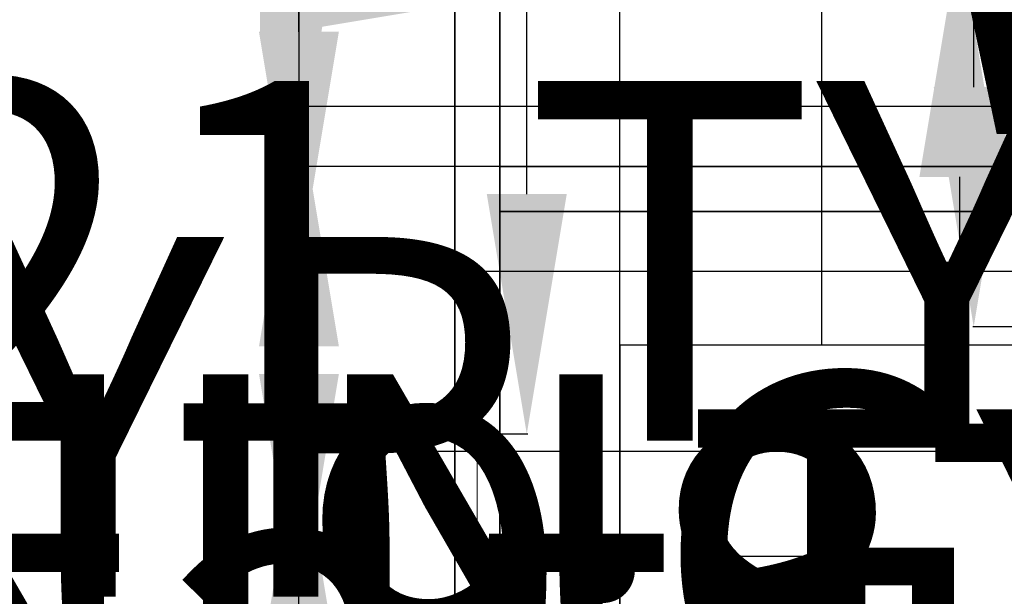
# Model space of a CAD drawing. Units: inches. Extents: x -307 to 2141, y -58 to 895.
# Tile 10 of 28: x 469 to 666, y 452 to 568. Entities that reach past the tile are written whole.
import ezdxf

# ---------------------------------------------------------------- set-up
doc = ezdxf.new("R2010")
doc.units = ezdxf.units.IN
doc.header["$MEASUREMENT"] = 0
for name, color, linetype, lineweight in [('A-ANNO-DIMS', 2, 'Continuous', 18), ('A-DOOR', 3, 'Continuous', 25), ('A-FLOR-CASE', 32, 'Continuous', 25), ('A-GLAZ', 4, 'Continuous', 18), ('A-WALL', 7, 'Continuous', 35)]:
    doc.layers.add(name, color=color, linetype=linetype, lineweight=lineweight)
doc.styles.get("Standard").update_dxf_attribs({"font": 'arial.ttf'})
doc.dimstyles.get("Standard").update_dxf_attribs({"dimtxt": 72, "dimasz": 48, "dimexe": 0.18, "dimexo": 0.0625, "dimgap": 0.09, "dimtad": 0, "dimtih": 1, "dimtoh": 1, "dimdec": 0, "dimrnd": 48, "dimzin": 0, "dimdsep": 46, "dimlunit": 3, "dimtxsty": 'Standard', "dimcen": 0.09, "dimadec": 0, "dimazin": 0, "dimtfac": 1, "dimtdec": 0, "dimtofl": 0, "dimtmove": 0, "dimatfit": 3, "dimfxl": 1, "dimtolj": 1, "dimtzin": 0, "dimarcsym": 0})

# ---------------------------------------------------------------- blocks, each defined once
blk = doc.blocks.new('*U3')
for p, q in [((-40, 0), (-40, 6)), ((0, 0), (0, 6))]:
    blk.add_line(p, q)
blk.add_lwpolyline([(0, 0), (-34.64, -20), (-35.52, -18.48), (-0.88, 1.52)], close=True)
blk.add_arc((0, 0), 40, 180, 210)
blk = doc.blocks.new('WIN-36IN')
for p, q in [((0, 36), (9, 36)), ((4.5, 0), (4.5, 36))]:
    blk.add_line(p, q)
blk.add_lwpolyline([(9, 36), (9, 0), (0, 0), (0, 36)])
blk = doc.blocks.new('*D26')
at = {"layer": 'A-ANNO-DIMS', "color": 0, "lineweight": -2, "transparency": 16777216}
for p, q in [((565.34, 584.2), (565.34, 572.08)), ((645.34, 584.2), (645.34, 572.08)), ((517.34, 572.26), (469.34, 572.26)), ((693.34, 572.26), (741.34, 572.26))]:
    blk.add_line(p, q, dxfattribs=at)
at = {"layer": 'A-ANNO-DIMS', "color": 0, "transparency": 16777216}
for points in [[(517.34, 580.26), (517.34, 564.26), (565.34, 572.26)], [(693.34, 580.26), (693.34, 564.26), (645.34, 572.26)]]:
    blk.add_solid(points, dxfattribs=at)
at = {"layer": 'Defpoints', "color": 0, "transparency": 16777216}
for p in [(565.34, 584.26), (645.34, 584.26), (565.34, 572.26)]:
    blk.add_point(p, dxfattribs=at)
at = {"layer": 'A-ANNO-DIMS', "color": 0, "transparency": 16777216, "insert": (178.23, 572.26), "char_height": 72, "attachment_point": 5}
blk.add_mtext('\\A1;BED 80 TYP.', dxfattribs=at)
blk = doc.blocks.new('*D27')
at = {"layer": 'A-ANNO-DIMS', "color": 0, "lineweight": -2, "transparency": 16777216}
for p, q in [((657.34, 692.26), (657.34, 740.26)), ((645.4, 644.26), (657.52, 644.26)), ((645.4, 584.26), (657.52, 584.26)), ((657.34, 536.26), (657.34, 488.26)), ((657.34, 488.26), (609.34, 488.26))]:
    blk.add_line(p, q, dxfattribs=at)
at = {"layer": 'A-ANNO-DIMS', "color": 0, "transparency": 16777216}
for points in [[(649.34, 692.26), (665.34, 692.26), (657.34, 644.26)], [(649.34, 536.26), (665.34, 536.26), (657.34, 584.26)]]:
    blk.add_solid(points, dxfattribs=at)
at = {"layer": 'Defpoints', "color": 0, "transparency": 16777216}
for p in [(645.34, 644.26), (645.34, 584.26), (657.34, 584.26)]:
    blk.add_point(p, dxfattribs=at)
at = {"layer": 'A-ANNO-DIMS', "color": 0, "transparency": 16777216, "insert": (433.81, 488.26), "char_height": 72, "attachment_point": 5}
blk.add_mtext('\\A1;60 TYP.', dxfattribs=at)
blk = doc.blocks.new('*D29')
at = {"layer": 'A-ANNO-DIMS', "color": 0, "lineweight": -2, "transparency": 16777216}
for p, q in [((747.42, 450.87), (699.42, 450.87)), ((795.42, 433.61), (795.42, 451.05)), ((882.03, 433.61), (882.03, 451.05)), ((930.03, 450.87), (978.03, 450.87))]:
    blk.add_line(p, q, dxfattribs=at)
at = {"layer": 'A-ANNO-DIMS', "color": 0, "transparency": 16777216}
for points in [[(747.42, 458.87), (747.42, 442.87), (795.42, 450.87)], [(930.03, 458.87), (930.03, 442.87), (882.03, 450.87)]]:
    blk.add_solid(points, dxfattribs=at)
at = {"layer": 'Defpoints', "color": 0, "transparency": 16777216}
for p in [(795.42, 450.87), (795.42, 433.55), (882.03, 433.55)]:
    blk.add_point(p, dxfattribs=at)
at = {"layer": 'A-ANNO-DIMS', "color": 0, "transparency": 16777216, "insert": (647.71, 450.87), "char_height": 72, "attachment_point": 5}
blk.add_mtext('\\A1;87', dxfattribs=at)
blk = doc.blocks.new('*D30')
at = {"layer": 'A-ANNO-DIMS', "color": 0, "lineweight": -2, "transparency": 16777216}
for p, q in [((570.74, 532.83), (570.74, 580.83)), ((570.74, 580.83), (618.74, 580.83)), ((565.4, 484.83), (570.92, 484.83)), ((565.4, 448.83), (570.92, 448.83)), ((570.74, 400.83), (570.74, 352.83))]:
    blk.add_line(p, q, dxfattribs=at)
at = {"layer": 'A-ANNO-DIMS', "color": 0, "transparency": 16777216}
for points in [[(562.74, 532.83), (578.74, 532.83), (570.74, 484.83)], [(562.74, 400.83), (578.74, 400.83), (570.74, 448.83)]]:
    blk.add_solid(points, dxfattribs=at)
at = {"layer": 'Defpoints', "color": 0, "transparency": 16777216}
for p in [(565.34, 484.83), (570.74, 484.83), (565.34, 448.83)]:
    blk.add_point(p, dxfattribs=at)
at = {"layer": 'A-ANNO-DIMS', "color": 0, "transparency": 16777216, "insert": (1030.17, 580.83), "char_height": 72, "attachment_point": 5}
blk.add_mtext('\\A1;WINDOW 36 TYP.', dxfattribs=at)
blk = doc.blocks.new('*D31')
at = {"layer": 'A-ANNO-DIMS', "color": 0, "lineweight": -2, "transparency": 16777216}
for p, q in [((556.34, 448.77), (556.34, 443.25)), ((565.34, 448.77), (565.34, 443.25)), ((508.34, 443.43), (460.34, 443.43)), ((613.34, 443.43), (661.34, 443.43))]:
    blk.add_line(p, q, dxfattribs=at)
at = {"layer": 'A-ANNO-DIMS', "color": 0, "transparency": 16777216}
for points in [[(508.34, 451.43), (508.34, 435.43), (556.34, 443.43)], [(613.34, 451.43), (613.34, 435.43), (565.34, 443.43)]]:
    blk.add_solid(points, dxfattribs=at)
at = {"layer": 'Defpoints', "color": 0, "transparency": 16777216}
for p in [(556.34, 448.83), (565.34, 448.83), (565.34, 443.43)]:
    blk.add_point(p, dxfattribs=at)
at = {"layer": 'A-ANNO-DIMS', "color": 0, "transparency": 16777216, "insert": (808.69, 443.43), "char_height": 72, "attachment_point": 5}
blk.add_mtext('\\A1;9 TYP.', dxfattribs=at)
blk = doc.blocks.new('*D35')
at = {"layer": 'A-ANNO-DIMS', "color": 0, "lineweight": -2, "transparency": 16777216}
for p, q in [((859.34, 453.77), (811.34, 453.77)), ((907.34, 443.03), (907.34, 453.95)), ((916.34, 443.03), (916.34, 453.95)), ((964.34, 453.77), (1012.34, 453.77))]:
    blk.add_line(p, q, dxfattribs=at)
at = {"layer": 'A-ANNO-DIMS', "color": 0, "transparency": 16777216}
for points in [[(859.34, 461.77), (859.34, 445.77), (907.34, 453.77)], [(964.34, 461.77), (964.34, 445.77), (916.34, 453.77)]]:
    blk.add_solid(points, dxfattribs=at)
at = {"layer": 'Defpoints', "color": 0, "transparency": 16777216}
for p in [(907.34, 453.77), (907.34, 442.97), (916.34, 442.97)]:
    blk.add_point(p, dxfattribs=at)
at = {"layer": 'A-ANNO-DIMS', "color": 0, "transparency": 16777216, "insert": (663.98, 453.77), "char_height": 72, "attachment_point": 5}
blk.add_mtext('\\A1;9 TYP.', dxfattribs=at)
blk = doc.blocks.new('*D36')
at = {"layer": 'A-ANNO-DIMS', "color": 0, "lineweight": -2, "transparency": 16777216}
for p, q in [((871.71, 562.4), (871.76, 610.4)), ((876.55, 514.4), (871.47, 514.4)), ((876.51, 481.35), (871.44, 481.36)), ((871.56, 433.36), (871.51, 385.36)), ((871.51, 385.36), (823.51, 385.36))]:
    blk.add_line(p, q, dxfattribs=at)
at = {"layer": 'A-ANNO-DIMS', "color": 0, "transparency": 16777216}
for points in [[(863.71, 562.41), (879.71, 562.4), (871.65, 514.4)], [(863.56, 433.37), (879.56, 433.35), (871.62, 481.36)]]:
    blk.add_solid(points, dxfattribs=at)
at = {"layer": 'Defpoints', "color": 0, "transparency": 16777216}
for p in [(876.61, 514.4), (871.62, 481.36), (876.57, 481.35)]:
    blk.add_point(p, dxfattribs=at)
at = {"layer": 'A-ANNO-DIMS', "color": 0, "transparency": 16777216, "insert": (548.95, 385.36), "char_height": 72, "attachment_point": 5}
blk.add_mtext('\\A1;WC 33 TYP.', dxfattribs=at)
blk = doc.blocks.new('*D37')
at = {"layer": 'A-ANNO-DIMS', "color": 0, "lineweight": -2, "transparency": 16777216}
for p, q in [((828.62, 519.41), (780.62, 519.46)), ((876.61, 514.46), (876.62, 519.54)), ((897.61, 514.44), (897.62, 519.51)), ((945.62, 519.28), (993.62, 519.22))]:
    blk.add_line(p, q, dxfattribs=at)
at = {"layer": 'A-ANNO-DIMS', "color": 0, "transparency": 16777216}
for points in [[(828.63, 527.41), (828.61, 511.41), (876.62, 519.36)], [(945.63, 527.28), (945.61, 511.28), (897.62, 519.33)]]:
    blk.add_solid(points, dxfattribs=at)
at = {"layer": 'Defpoints', "color": 0, "transparency": 16777216}
for p in [(876.62, 519.36), (876.61, 514.4), (897.61, 514.38)]:
    blk.add_point(p, dxfattribs=at)
at = {"layer": 'A-ANNO-DIMS', "color": 0, "transparency": 16777216, "insert": (604.68, 519.46), "char_height": 72, "attachment_point": 5}
blk.add_mtext('\\A1;21 TYP.', dxfattribs=at)
blk = doc.blocks.new('*D51')
at = {"layer": 'A-ANNO-DIMS', "color": 0, "lineweight": -2, "transparency": 16777216}
for p, q in [((562.8, 379.11), (562.8, 427.11)), ((562.8, 427.11), (610.8, 427.11)), ((565.27, 331.11), (562.62, 331.11)), ((565.27, 315.87), (562.62, 315.87)), ((562.8, 267.87), (562.8, 219.87))]:
    blk.add_line(p, q, dxfattribs=at)
at = {"layer": 'A-ANNO-DIMS', "color": 0, "transparency": 16777216}
for points in [[(554.8, 379.11), (570.8, 379.11), (562.8, 331.11)], [(554.8, 267.87), (570.8, 267.87), (562.8, 315.87)]]:
    blk.add_solid(points, dxfattribs=at)
at = {"layer": 'Defpoints', "color": 0, "transparency": 16777216}
for p in [(562.8, 331.11), (565.34, 331.11), (565.34, 315.87)]:
    blk.add_point(p, dxfattribs=at)
at = {"layer": 'A-ANNO-DIMS', "color": 0, "transparency": 16777216, "insert": (659.34, 427.11), "char_height": 72, "attachment_point": 5}
blk.add_mtext('\\A1;15', dxfattribs=at)
blk = doc.blocks.new('*D52')
at = {"layer": 'A-ANNO-DIMS', "color": 0, "lineweight": -2, "transparency": 16777216}
for p, q in [((660.21, 554.25), (660.21, 602.25)), ((673.8, 506.25), (660.03, 506.25)), ((673.8, 415.25), (660.03, 415.25)), ((660.21, 367.25), (660.21, 319.25))]:
    blk.add_line(p, q, dxfattribs=at)
at = {"layer": 'A-ANNO-DIMS', "color": 0, "transparency": 16777216}
for points in [[(652.21, 554.25), (668.21, 554.25), (660.21, 506.25)], [(652.21, 367.25), (668.21, 367.25), (660.21, 415.25)]]:
    blk.add_solid(points, dxfattribs=at)
at = {"layer": 'Defpoints', "color": 0, "transparency": 16777216}
for p in [(673.86, 506.25), (660.21, 415.25), (673.86, 415.25)]:
    blk.add_point(p, dxfattribs=at)
at = {"layer": 'A-ANNO-DIMS', "color": 0, "transparency": 16777216, "insert": (660.21, 460.75), "char_height": 72, "attachment_point": 5}
blk.add_mtext('\\A1;DINING SET 91', dxfattribs=at)
blk = doc.blocks.new('*D54')
at = {"layer": 'A-ANNO-DIMS', "color": 0, "lineweight": -2, "transparency": 16777216}
for p, q in [((605.34, 412.35), (605.34, 460.35)), ((605.34, 460.35), (653.34, 460.35)), ((596.4, 364.35), (605.52, 364.35)), ((596.4, 304.35), (605.52, 304.35)), ((605.34, 256.35), (605.34, 208.35))]:
    blk.add_line(p, q, dxfattribs=at)
at = {"layer": 'A-ANNO-DIMS', "color": 0, "transparency": 16777216}
for points in [[(597.34, 412.35), (613.34, 412.35), (605.34, 364.35)], [(597.34, 256.35), (613.34, 256.35), (605.34, 304.35)]]:
    blk.add_solid(points, dxfattribs=at)
at = {"layer": 'Defpoints', "color": 0, "transparency": 16777216}
for p in [(596.34, 364.35), (605.34, 364.35), (596.34, 304.35)]:
    blk.add_point(p, dxfattribs=at)
at = {"layer": 'A-ANNO-DIMS', "color": 0, "transparency": 16777216, "insert": (854, 460.35), "char_height": 72, "attachment_point": 5}
blk.add_mtext('\\A1;DESK 60', dxfattribs=at)
blk = doc.blocks.new('*D62')
at = {"layer": 'A-ANNO-DIMS', "color": 0, "lineweight": -2, "transparency": 16777216}
for p, q in [((556.34, 691.4), (556.34, 722.72)), ((604.34, 722.54), (656.85, 722.54)), ((868.34, 722.54), (815.82, 722.54)), ((916.34, 490.97), (916.34, 722.72))]:
    blk.add_line(p, q, dxfattribs=at)
at = {"layer": 'A-ANNO-DIMS', "color": 0, "transparency": 16777216}
for points in [[(604.34, 730.54), (604.34, 714.54), (556.34, 722.54)], [(868.34, 730.54), (868.34, 714.54), (916.34, 722.54)]]:
    blk.add_solid(points, dxfattribs=at)
at = {"layer": 'Defpoints', "color": 0, "transparency": 16777216}
for p in [(916.34, 722.54), (556.34, 691.34), (916.34, 490.9)]:
    blk.add_point(p, dxfattribs=at)
at = {"layer": 'A-ANNO-DIMS', "color": 0, "transparency": 16777216, "insert": (736.34, 722.54), "char_height": 72, "attachment_point": 5}
blk.add_mtext('\\A1;360', dxfattribs=at)
blk = doc.blocks.new('*D64')
at = {"layer": 'A-ANNO-DIMS', "color": 0, "lineweight": -2, "transparency": 16777216}
for p, q in [((556.27, 691.34), (524.95, 691.34)), ((525.13, 643.34), (525.13, 465.69)), ((525.13, 214.34), (525.13, 391.99)), ((556.27, 166.34), (524.95, 166.34))]:
    blk.add_line(p, q, dxfattribs=at)
at = {"layer": 'A-ANNO-DIMS', "color": 0, "transparency": 16777216}
for points in [[(517.13, 643.34), (533.13, 643.34), (525.13, 691.34)], [(517.13, 214.34), (533.13, 214.34), (525.13, 166.34)]]:
    blk.add_solid(points, dxfattribs=at)
at = {"layer": 'Defpoints', "color": 0, "transparency": 16777216}
for p in [(525.13, 691.34), (556.34, 691.34), (556.34, 166.34)]:
    blk.add_point(p, dxfattribs=at)
at = {"layer": 'A-ANNO-DIMS', "color": 0, "transparency": 16777216, "insert": (525.13, 428.84), "char_height": 72, "attachment_point": 5}
blk.add_mtext('\\A1;525', dxfattribs=at)
blk = doc.blocks.new('*D67')
at = {"layer": 'A-ANNO-DIMS', "color": 0, "lineweight": -2, "transparency": 16777216}
for p, q in [((525.13, 496.83), (525.13, 544.83)), ((556.27, 448.83), (524.95, 448.83)), ((556.27, 370.34), (524.95, 370.34)), ((525.13, 322.34), (525.13, 274.34))]:
    blk.add_line(p, q, dxfattribs=at)
at = {"layer": 'A-ANNO-DIMS', "color": 0, "transparency": 16777216}
for points in [[(517.13, 496.83), (533.13, 496.83), (525.13, 448.83)], [(517.13, 322.34), (533.13, 322.34), (525.13, 370.34)]]:
    blk.add_solid(points, dxfattribs=at)
at = {"layer": 'Defpoints', "color": 0, "transparency": 16777216}
for p in [(525.13, 448.83), (556.34, 448.83), (556.34, 370.34)]:
    blk.add_point(p, dxfattribs=at)
at = {"layer": 'A-ANNO-DIMS', "color": 0, "transparency": 16777216, "insert": (525.13, 409.59), "char_height": 72, "attachment_point": 5}
blk.add_mtext('\\A1;78.49', dxfattribs=at)
blk = doc.blocks.new('*D68')
at = {"layer": 'A-ANNO-DIMS', "color": 0, "lineweight": -2, "transparency": 16777216}
for p, q in [((525.13, 586.34), (525.13, 634.34)), ((525.13, 634.34), (573.13, 634.34)), ((565.27, 538.34), (524.95, 538.34)), ((556.27, 484.83), (524.95, 484.83)), ((525.13, 436.83), (525.13, 388.83))]:
    blk.add_line(p, q, dxfattribs=at)
at = {"layer": 'A-ANNO-DIMS', "color": 0, "transparency": 16777216}
for points in [[(517.13, 586.34), (533.13, 586.34), (525.13, 538.34)], [(517.13, 436.83), (533.13, 436.83), (525.13, 484.83)]]:
    blk.add_solid(points, dxfattribs=at)
at = {"layer": 'Defpoints', "color": 0, "transparency": 16777216}
for p in [(525.13, 538.34), (565.34, 538.34), (556.34, 484.83)]:
    blk.add_point(p, dxfattribs=at)
at = {"layer": 'A-ANNO-DIMS', "color": 0, "transparency": 16777216, "insert": (687.75, 634.34), "char_height": 72, "attachment_point": 5}
blk.add_mtext('\\A1;53.51', dxfattribs=at)
blk = doc.blocks.new('*D69')
at = {"layer": 'A-ANNO-DIMS', "color": 0, "lineweight": -2, "transparency": 16777216}
for p, q in [((525.13, 682.34), (525.13, 730.34)), ((525.13, 730.34), (573.13, 730.34)), ((565.27, 682.34), (524.95, 682.34)), ((525.13, 586.34), (525.13, 634.34)), ((565.27, 538.34), (524.95, 538.34))]:
    blk.add_line(p, q, dxfattribs=at)
at = {"layer": 'A-ANNO-DIMS', "color": 0, "transparency": 16777216}
for points in [[(517.13, 634.34), (533.13, 634.34), (525.13, 682.34)], [(517.13, 586.34), (533.13, 586.34), (525.13, 538.34)]]:
    blk.add_solid(points, dxfattribs=at)
at = {"layer": 'Defpoints', "color": 0, "transparency": 16777216}
for p in [(525.13, 682.34), (565.34, 682.34), (565.34, 538.34)]:
    blk.add_point(p, dxfattribs=at)
at = {"layer": 'A-ANNO-DIMS', "color": 0, "transparency": 16777216, "insert": (649.22, 730.34), "char_height": 72, "attachment_point": 5}
blk.add_mtext('\\A1;144', dxfattribs=at)
blk = doc.blocks.new('*D82')
at = {"layer": 'A-ANNO-DIMS', "color": 0, "lineweight": -2, "transparency": 16777216}
for p, q in [((525.13, 565.34), (525.13, 613.34)), ((525.13, 613.34), (573.13, 613.34)), ((802.27, 517.34), (524.95, 517.34)), ((802.27, 481.34), (524.95, 481.34)), ((525.13, 433.34), (525.13, 385.34))]:
    blk.add_line(p, q, dxfattribs=at)
at = {"layer": 'A-ANNO-DIMS', "color": 0, "transparency": 16777216}
for points in [[(517.13, 565.34), (533.13, 565.34), (525.13, 517.34)], [(517.13, 433.34), (533.13, 433.34), (525.13, 481.34)]]:
    blk.add_solid(points, dxfattribs=at)
at = {"layer": 'Defpoints', "color": 0, "transparency": 16777216}
for p in [(525.13, 517.34), (802.34, 517.34), (802.34, 481.34)]:
    blk.add_point(p, dxfattribs=at)
at = {"layer": 'A-ANNO-DIMS', "color": 0, "transparency": 16777216, "insert": (624.74, 613.34), "char_height": 72, "attachment_point": 5}
blk.add_mtext('\\A1;36', dxfattribs=at)
blk = doc.blocks.new('*D83')
at = {"layer": 'A-ANNO-DIMS', "color": 0, "lineweight": -2, "transparency": 16777216}
for p, q in [((947.54, 538.9), (947.54, 586.9)), ((916.4, 490.9), (947.72, 490.9)), ((907.4, 481.34), (947.72, 481.34)), ((947.54, 433.34), (947.54, 385.34)), ((947.54, 385.34), (899.54, 385.34))]:
    blk.add_line(p, q, dxfattribs=at)
at = {"layer": 'A-ANNO-DIMS', "color": 0, "transparency": 16777216}
for points in [[(939.54, 538.9), (955.54, 538.9), (947.54, 490.9)], [(939.54, 433.34), (955.54, 433.34), (947.54, 481.34)]]:
    blk.add_solid(points, dxfattribs=at)
at = {"layer": 'Defpoints', "color": 0, "transparency": 16777216}
for p in [(916.34, 490.9), (907.34, 481.34), (947.54, 481.34)]:
    blk.add_point(p, dxfattribs=at)
at = {"layer": 'A-ANNO-DIMS', "color": 0, "transparency": 16777216, "insert": (777.97, 385.34), "char_height": 72, "attachment_point": 5}
blk.add_mtext('\\A1;9.563', dxfattribs=at)
blk = doc.blocks.new('*D87')
at = {"layer": 'A-ANNO-DIMS', "color": 0, "lineweight": -2, "transparency": 16777216}
for p, q in [((525.13184, 448.340828), (525.13184, 496.340828)), ((625.27334, 400.340828), (524.95184, 400.340828)), ((625.27334, 304.340828), (524.95184, 304.340828)), ((525.13184, 256.340828), (525.13184, 208.340828))]:
    blk.add_line(p, q, dxfattribs=at)
at = {"layer": 'A-ANNO-DIMS', "color": 0, "transparency": 16777216}
for points in [[(517.13184, 448.340828), (533.13184, 448.340828), (525.13184, 400.340828)], [(517.13184, 256.340828), (533.13184, 256.340828), (525.13184, 304.340828)]]:
    blk.add_solid(points, dxfattribs=at)
at = {"layer": 'Defpoints', "color": 0, "transparency": 16777216}
for p in [(525.13184, 400.340828), (625.33584, 400.340828), (625.33584, 304.340828)]:
    blk.add_point(p, dxfattribs=at)
at = {"layer": 'A-ANNO-DIMS', "color": 0, "transparency": 16777216, "insert": (525.13184, 352.340828), "char_height": 72, "attachment_point": 5}
blk.add_mtext('\\A1;96', dxfattribs=at)
blk = doc.blocks.new('*D88')
at = {"layer": 'A-ANNO-DIMS', "color": 0, "lineweight": -2, "transparency": 16777216}
for p, q in [((517.33584, 722.544828), (469.33584, 722.544828)), ((565.33584, 295.403328), (565.33584, 722.724828)), ((754.33584, 271.403328), (754.33584, 722.724828)), ((802.33584, 722.544828), (850.33584, 722.544828))]:
    blk.add_line(p, q, dxfattribs=at)
at = {"layer": 'A-ANNO-DIMS', "color": 0, "transparency": 16777216}
for points in [[(517.33584, 730.544828), (517.33584, 714.544828), (565.33584, 722.544828)], [(802.33584, 730.544828), (802.33584, 714.544828), (754.33584, 722.544828)]]:
    blk.add_solid(points, dxfattribs=at)
at = {"layer": 'Defpoints', "color": 0, "transparency": 16777216}
for p in [(754.33584, 722.544828), (565.33584, 295.340828), (754.33584, 271.340828)]:
    blk.add_point(p, dxfattribs=at)
at = {"layer": 'A-ANNO-DIMS', "color": 0, "transparency": 16777216, "insert": (659.83584, 722.544828), "char_height": 72, "attachment_point": 5}
blk.add_mtext('\\A1;189', dxfattribs=at)
blk = doc.blocks.new('*D94')
at = {"layer": 'A-ANNO-DIMS', "color": 0, "lineweight": -2, "transparency": 16777216}
for p, q in [((517.34, 722.54), (469.34, 722.54)), ((565.34, 529.4), (565.34, 722.72)), ((629.84, 529.4), (629.84, 722.72)), ((677.84, 722.54), (725.84, 722.54))]:
    blk.add_line(p, q, dxfattribs=at)
at = {"layer": 'A-ANNO-DIMS', "color": 0, "transparency": 16777216}
for points in [[(517.34, 730.54), (517.34, 714.54), (565.34, 722.54)], [(677.84, 730.54), (677.84, 714.54), (629.84, 722.54)]]:
    blk.add_solid(points, dxfattribs=at)
at = {"layer": 'Defpoints', "color": 0, "transparency": 16777216}
for p in [(629.84, 722.54), (565.34, 529.34), (629.84, 529.34)]:
    blk.add_point(p, dxfattribs=at)
at = {"layer": 'A-ANNO-DIMS', "color": 0, "transparency": 16777216, "insert": (819.9, 722.54), "char_height": 72, "attachment_point": 5}
blk.add_mtext('\\A1;64.5', dxfattribs=at)
blk = doc.blocks.new('*D95')
at = {"layer": 'A-ANNO-DIMS', "color": 0, "lineweight": -2, "transparency": 16777216}
for p, q in [((947.54, 577.34), (947.54, 625.34)), ((947.54, 625.34), (995.54, 625.34)), ((629.9, 529.34), (947.72, 529.34)), ((629.9, 502.66), (947.72, 502.66)), ((947.54, 454.66), (947.54, 406.66))]:
    blk.add_line(p, q, dxfattribs=at)
at = {"layer": 'A-ANNO-DIMS', "color": 0, "transparency": 16777216}
for points in [[(939.54, 577.34), (955.54, 577.34), (947.54, 529.34)], [(939.54, 454.66), (955.54, 454.66), (947.54, 502.66)]]:
    blk.add_solid(points, dxfattribs=at)
at = {"layer": 'Defpoints', "color": 0, "transparency": 16777216}
for p in [(629.84, 529.34), (947.54, 529.34), (629.84, 502.66)]:
    blk.add_point(p, dxfattribs=at)
at = {"layer": 'A-ANNO-DIMS', "color": 0, "transparency": 16777216, "insert": (1117.8, 625.34), "char_height": 72, "attachment_point": 5}
blk.add_mtext('\\A1;26.68', dxfattribs=at)
blk = doc.blocks.new('*D98')
at = {"layer": 'A-ANNO-DIMS', "color": 0, "lineweight": -2, "transparency": 16777216}
for p, q in [((525.13, 637.34), (525.13, 685.34)), ((525.13, 685.34), (573.13, 685.34)), ((787.27, 589.34), (524.95, 589.34)), ((787.27, 550.34), (524.95, 550.34)), ((525.13, 502.34), (525.13, 454.34))]:
    blk.add_line(p, q, dxfattribs=at)
at = {"layer": 'A-ANNO-DIMS', "color": 0, "transparency": 16777216}
for points in [[(517.13, 637.34), (533.13, 637.34), (525.13, 589.34)], [(517.13, 502.34), (533.13, 502.34), (525.13, 550.34)]]:
    blk.add_solid(points, dxfattribs=at)
at = {"layer": 'Defpoints', "color": 0, "transparency": 16777216}
for p in [(525.13, 589.34), (787.34, 589.34), (787.34, 550.34)]:
    blk.add_point(p, dxfattribs=at)
at = {"layer": 'A-ANNO-DIMS', "color": 0, "transparency": 16777216, "insert": (624.84, 685.34), "char_height": 72, "attachment_point": 5}
blk.add_mtext('\\A1;39', dxfattribs=at)
blk = doc.blocks.new('*D107')
at = {"layer": 'A-ANNO-DIMS', "color": 0, "lineweight": -2, "transparency": 16777216}
for p, q in [((517.34, 722.54), (469.34, 722.54)), ((565.34, 409.4), (565.34, 722.72)), ((589.34, 409.4), (589.34, 722.72)), ((637.34, 722.54), (685.34, 722.54))]:
    blk.add_line(p, q, dxfattribs=at)
at = {"layer": 'A-ANNO-DIMS', "color": 0, "transparency": 16777216}
for points in [[(517.34, 730.54), (517.34, 714.54), (565.34, 722.54)], [(637.34, 730.54), (637.34, 714.54), (589.34, 722.54)]]:
    blk.add_solid(points, dxfattribs=at)
at = {"layer": 'Defpoints', "color": 0, "transparency": 16777216}
for p in [(589.34, 722.54), (565.34, 409.34), (589.34, 409.34)]:
    blk.add_point(p, dxfattribs=at)
at = {"layer": 'A-ANNO-DIMS', "color": 0, "transparency": 16777216, "insert": (835.49, 722.54), "char_height": 72, "attachment_point": 5}
blk.add_mtext('\\A1;24.003', dxfattribs=at)
blk = doc.blocks.new('*D108')
at = {"layer": 'A-ANNO-DIMS', "color": 0, "lineweight": -2, "transparency": 16777216}
for p, q in [((947.54, 550.66), (947.54, 598.66)), ((589.4, 502.66), (947.72, 502.66)), ((589.4, 409.34), (947.72, 409.34)), ((947.54, 361.34), (947.54, 313.34))]:
    blk.add_line(p, q, dxfattribs=at)
at = {"layer": 'A-ANNO-DIMS', "color": 0, "transparency": 16777216}
for points in [[(939.54, 550.66), (955.54, 550.66), (947.54, 502.66)], [(939.54, 361.34), (955.54, 361.34), (947.54, 409.34)]]:
    blk.add_solid(points, dxfattribs=at)
at = {"layer": 'Defpoints', "color": 0, "transparency": 16777216}
for p in [(589.34, 502.66), (947.54, 502.66), (589.34, 409.34)]:
    blk.add_point(p, dxfattribs=at)
at = {"layer": 'A-ANNO-DIMS', "color": 0, "transparency": 16777216, "insert": (947.54, 456), "char_height": 72, "attachment_point": 5}
blk.add_mtext('\\A1;93.32', dxfattribs=at)

msp = doc.modelspace()

# ---------------------------------------------------------------- linework, layer by layer
at = {"layer": 'A-FLOR-CASE'}
for points in [[(589.339, 502.6632), (589.339, 409.3408), (565.3358, 409.3408), (565.3358, 529.3408), (589.339, 529.3408)], [(589.339, 502.6632), (629.8358, 502.6632), (629.8358, 529.3408), (565.3358, 529.3408), (565.3358, 502.6632)]]:
    msp.add_lwpolyline(points, dxfattribs=at)
at = {"layer": 'A-WALL'}
for p, q in [((556.3358, 691.3408), (556.3358, 91.3408)), ((565.3358, 682.3408), (565.3358, 100.3408)), ((694.3358, 538.3408), (565.3358, 538.3408)), ((694.3358, 529.3408), (565.3358, 529.3408))]:
    msp.add_line(p, q, dxfattribs=at)

# ---------------------------------------------------------------- block references
at = {"layer": 'A-DOOR', "xscale": 1.272826874134829, "yscale": 1.272826874134829, "zscale": 1.272826874134829, "rotation": 270}
msp.add_blockref('*U3', (686.6989, 538.3408), dxfattribs=at)
at = {"layer": 'A-GLAZ'}
msp.add_blockref('WIN-36IN', (556.336, 448.8337), dxfattribs=at)

# ---------------------------------------------------------------- dimensions: what is measured, and where the dimension line sits
at = {"layer": 'A-ANNO-DIMS'}
for base, p1, p2, angle, override, picture, middle in [((525.1318, 682.3408), (565.3358, 538.3408), (565.3358, 682.3408), 90, {"dimdec": 0, "dimlfac": 1, "dimrnd": 0, "dimzin": 0, "dimdsep": 46, "dimlunit": 2}, '*D69', (649.2246, 730.3408)), ((525.1318, 589.3408), (787.3358, 550.3408), (787.3358, 589.3408), 90, {"dimdec": 0, "dimlfac": 1, "dimrnd": 0, "dimzin": 0, "dimdsep": 46, "dimlunit": 2}, '*D98', (624.8398, 685.3408)), ((525.1318, 691.3408), (556.3358, 166.3408), (556.3358, 691.3408), 90, {"dimdec": 0, "dimlfac": 1, "dimrnd": 0, "dimzin": 0, "dimdsep": 46, "dimlunit": 2}, '*D64', (525.1318, 428.8408)), ((525.1318, 538.3408), (556.3358, 484.8333), (565.3358, 538.3408), 90, {"dimdec": 2, "dimlfac": 1, "dimrnd": 0, "dimzin": 0, "dimdsep": 46, "dimlunit": 2}, '*D68', (687.7539, 634.3408)), ((947.5398, 529.3408), (629.8358, 502.6632), (629.8358, 529.3408), 90, {"dimdec": 2, "dimlfac": 1, "dimrnd": 0, "dimzin": 0, "dimdsep": 46, "dimlunit": 2}, '*D95', (1117.799, 625.3408)), ((525.1318, 517.3408), (802.3358, 481.3408), (802.3358, 517.3408), 90, {"dimdec": 0, "dimlfac": 1, "dimrnd": 0, "dimzin": 0, "dimdsep": 46, "dimlunit": 2}, '*D82', (624.7416, 613.3408)), ((947.5398, 502.6632), (589.339, 409.3408), (589.339, 502.6632), 90, {"dimdec": 2, "dimlfac": 1, "dimrnd": 0, "dimzin": 0, "dimdsep": 46, "dimlunit": 2}, '*D108', (947.5398, 456.002)), ((947.5398, 481.3408), (916.3358, 490.9034), (907.3358, 481.3408), 90, {"dimdec": 3, "dimlfac": 1, "dimrnd": 0, "dimzin": 0, "dimdsep": 46, "dimlunit": 2}, '*D83', (777.9683, 385.3408)), ((525.1318, 448.8333), (556.3358, 370.3416), (556.3358, 448.8333), 90, {"dimdec": 2, "dimlfac": 1, "dimrnd": 0, "dimzin": 0, "dimdsep": 46, "dimlunit": 2}, '*D67', (525.1318, 409.5874)), ((795.4208, 450.8711), (882.0282, 433.5496), (795.4208, 433.5496), 180, {"dimdec": 0, "dimlfac": 1, "dimrnd": 0, "dimzin": 0, "dimdsep": 46, "dimlunit": 2}, '*D29', (647.7128, 450.8711)), ((525.1318, 400.3408), (625.3358, 304.3408), (625.3358, 400.3408), 90, {"dimdec": 0, "dimlfac": 1, "dimrnd": 0, "dimzin": 0, "dimdsep": 46, "dimlunit": 2}, '*D87', (525.1318, 352.3408)), ((562.7955, 331.1086), (565.3358, 315.8666), (565.3358, 331.1086), 90, {"dimdec": 0, "dimlfac": 1, "dimrnd": 0, "dimzin": 0, "dimdsep": 46, "dimlunit": 2}, '*D51', (659.3357, 427.1086))]:
    dim = msp.add_linear_dim(base=base, p1=p1, p2=p2, angle=angle, dimstyle='Standard', override=override, dxfattribs=at)
    dim.commit()
    dim.dimension.update_dxf_attribs({"geometry": picture, "text_midpoint": middle})
for base, p1, p2, override, picture, middle in [((754.3358, 722.5448), (565.3358, 295.3408), (754.3358, 271.3408), {"dimdec": 0, "dimlfac": 1, "dimrnd": 0, "dimzin": 0, "dimdsep": 46, "dimlunit": 2}, '*D88', (659.8358, 722.5448)), ((629.8358, 722.5448), (565.3358, 529.3408), (629.8358, 529.3408), {"dimdec": 1, "dimlfac": 1, "dimrnd": 0, "dimzin": 0, "dimdsep": 46, "dimlunit": 2}, '*D94', (819.904, 722.5448)), ((589.339, 722.5448), (565.3358, 409.3408), (589.339, 409.3408), {"dimdec": 3, "dimlfac": 1, "dimrnd": 0, "dimzin": 0, "dimdsep": 46, "dimlunit": 2}, '*D107', (835.4945, 722.5448)), ((916.3358, 722.5448), (556.3358, 691.3408), (916.3358, 490.9034), {"dimdec": 0, "dimlfac": 1, "dimrnd": 0, "dimzin": 0, "dimdsep": 46, "dimlunit": 2}, '*D62', (736.3358, 722.5448))]:
    dim = msp.add_linear_dim(base=base, p1=p1, p2=p2, dimstyle='Standard', override=override, dxfattribs=at)
    dim.commit()
    dim.dimension.update_dxf_attribs({"geometry": picture, "text_midpoint": middle})
for base, p1, p2, angle, text, picture, middle in [((570.7358, 484.8333), (565.3358, 448.8333), (565.3358, 484.8333), 90, 'WINDOW <> TYP.', '*D30', (1030.1737, 580.8333)), ((565.3358, 572.2648), (645.3359, 584.2648), (565.3358, 584.2648), 180, 'BED <> TYP.', '*D26', (178.2254, 572.2648)), ((657.3359, 584.2648), (645.3359, 644.2648), (645.3359, 584.2648), 270, '<> TYP.', '*D27', (433.8134, 488.2648)), ((660.2083, 415.2485), (673.8583, 506.2485), (673.8583, 415.2485), 270, 'DINING SET <>', '*D52', (660.2083, 460.7485)), ((876.6162, 519.3557), (897.6106, 514.3753), (876.6106, 514.3988), 179.935892, '<> TYP.', '*D37', (604.6763, 519.4631)), ((871.6167, 481.3581), (876.6106, 514.3988), (876.5736, 481.3526), 269.935892, 'WC <> TYP.', '*D36', (548.95, 385.3582)), ((605.3358, 364.3488), (596.3358, 304.3488), (596.3358, 364.3488), 90, 'DESK <>', '*D54', (854.0043, 460.3488)), ((907.3358, 453.7692), (916.3358, 442.9669), (907.3358, 442.9669), 180, '<> TYP.', '*D35', (663.9798, 453.7692))]:
    dim = msp.add_linear_dim(base=base, p1=p1, p2=p2, angle=angle, text=text, dimstyle='Standard', override={"dimdec": 0, "dimlfac": 1, "dimrnd": 0, "dimzin": 0, "dimdsep": 46, "dimlunit": 2}, dxfattribs=at)
    dim.commit()
    dim.dimension.update_dxf_attribs({"geometry": picture, "text_midpoint": middle})
dim = msp.add_linear_dim(base=(565.3358, 443.4333), p1=(556.3358, 448.8333), p2=(565.3358, 448.8333), text='<> TYP.', dimstyle='Standard', override={"dimdec": 0, "dimlfac": 1, "dimrnd": 0, "dimzin": 0, "dimdsep": 46, "dimlunit": 2}, dxfattribs=at)
dim.commit()
dim.dimension.update_dxf_attribs({"geometry": '*D31', "text_midpoint": (808.6919, 443.4333)})

doc.saveas('drawing.dxf')
